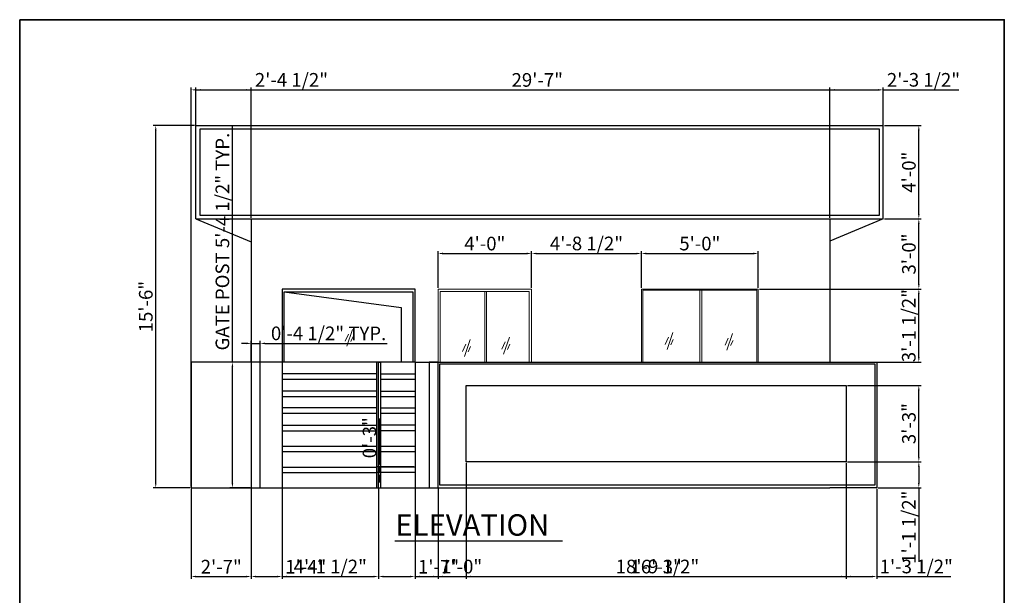
# Model space of a CAD drawing. Units: inches. Extents: x 1484 to 2008, y 1843 to 2590.
# Tile 21 of 21: x 1484 to 1990, y 2295 to 2590. Entities that reach past the tile are written whole.
import ezdxf

# ---------------------------------------------------------------- set-up
doc = ezdxf.new("R2010")
doc.units = ezdxf.units.IN
for name, color, linetype, lineweight in [('A-ANNO-DIMS', 2, 'Continuous', 18), ('A-ANNO-TEXT', 7, 'Continuous', 25), ('A-ANNO-TTLB', 7, 'Continuous', 35), ('A-ELEV', 7, 'Continuous', 30), ('A-ELEV-DOOR', 4, 'Continuous', 25), ('A-ELEV-GATE', 7, 'Continuous', 25), ('A-ELEV-GLAZ', 4, 'Continuous', 18), ('A-ELEV-ROOF', 7, 'Continuous', 30)]:
    doc.layers.add(name, color=color, linetype=linetype, lineweight=lineweight)
doc.styles.get("Standard").update_dxf_attribs({"font": 'arial.ttf'})
doc.dimstyles.new('ISO-25', dxfattribs={"dimtxt": 7, "dimasz": 2.5, "dimexe": 1.25, "dimexo": 0.625, "dimtad": 1, "dimdec": 0, "dimlunit": 3, "dimtxsty": 'Standard', "dimcen": 2.5, "dimadec": 0, "dimazin": 0, "dimtfac": 1, "dimtdec": 0, "dimtmove": 0, "dimatfit": 3, "dimfxl": 1, "dimarcsym": 0})

# ---------------------------------------------------------------- blocks, each defined once
blk = doc.blocks.new('GLASS-REFLECTION')
for p, q in [((1.68, 6.24), (0, 2.6)), ((3.87, 8.69), (0.89, 0)), ((4.11, 5.06), (2.86, 2.41))]:
    blk.add_line(p, q)
blk = doc.blocks.new('GATE-POST-ELEV')
blk.add_lwpolyline([(4.59, 64.44), (0, 64.44), (0, 0), (4.59, 0)], close=True)
blk = doc.blocks.new('*D15')
at = {"layer": 'A-ANNO-DIMS', "color": 0, "lineweight": -2, "transparency": 16777216}
for p, q in [((1593.25, 2414.26), (1593.25, 2535.55)), ((1602.29, 2414.26), (1592, 2414.26)), ((1593.25, 2352.32), (1593.25, 2411.76)), ((1602.29, 2349.82), (1592, 2349.82))]:
    blk.add_line(p, q, dxfattribs=at)
at = {"layer": 'A-ANNO-DIMS', "color": 0, "transparency": 16777216}
for points in [[(1592.84, 2411.76), (1593.67, 2411.76), (1593.25, 2414.26)], [(1592.84, 2352.32), (1593.67, 2352.32), (1593.25, 2349.82)]]:
    blk.add_solid(points, dxfattribs=at)
at = {"layer": 'Defpoints', "color": 0, "transparency": 16777216}
for p in [(1593.25, 2414.26), (1602.92, 2414.26), (1602.92, 2349.82)]:
    blk.add_point(p, dxfattribs=at)
at = {"layer": 'A-ANNO-DIMS', "color": 0, "transparency": 16777216, "insert": (1589.01, 2476.16), "char_height": 7, "attachment_point": 5, "rotation": 90}
blk.add_mtext('GATE POST 5\'-4 1/2" TYP.', dxfattribs=at)
blk = doc.blocks.new('*D16')
at = {"layer": 'A-ANNO-DIMS', "color": 0, "lineweight": -2, "transparency": 16777216}
for p, q in [((1600.42, 2423.92), (1597.92, 2423.92)), ((1602.92, 2414.88), (1602.92, 2425.17)), ((1602.92, 2423.92), (1607.51, 2423.92)), ((1607.51, 2414.88), (1607.51, 2425.17)), ((1610.01, 2423.92), (1672.74, 2423.92))]:
    blk.add_line(p, q, dxfattribs=at)
at = {"layer": 'A-ANNO-DIMS', "color": 0, "transparency": 16777216}
for points in [[(1600.42, 2424.34), (1600.42, 2423.5), (1602.92, 2423.92)], [(1610.01, 2424.34), (1610.01, 2423.5), (1607.51, 2423.92)]]:
    blk.add_solid(points, dxfattribs=at)
at = {"layer": 'Defpoints', "color": 0, "transparency": 16777216}
for p in [(1607.51, 2423.92), (1602.92, 2414.26), (1607.51, 2414.26)]:
    blk.add_point(p, dxfattribs=at)
at = {"layer": 'A-ANNO-DIMS', "color": 0, "transparency": 16777216, "insert": (1642.62, 2428.17), "char_height": 7, "attachment_point": 5}
blk.add_mtext('0\'-4 1/2" TYP.', dxfattribs=at)
blk = doc.blocks.new('*D44')
at = {"layer": 'A-ANNO-DIMS', "color": 0, "lineweight": -2, "transparency": 16777216}
for p, q in [((1572.14, 2350.44), (1572.14, 2555.32)), ((1574.64, 2554.07), (1924.89, 2554.07)), ((1927.39, 2536.44), (1927.39, 2555.32))]:
    blk.add_line(p, q, dxfattribs=at)
at = {"layer": 'A-ANNO-DIMS', "color": 0, "transparency": 16777216}
for points in [[(1574.64, 2554.49), (1574.64, 2553.65), (1572.14, 2554.07)], [(1924.89, 2554.49), (1924.89, 2553.65), (1927.39, 2554.07)]]:
    blk.add_solid(points, dxfattribs=at)
at = {"layer": 'Defpoints', "color": 0, "transparency": 16777216}
for p in [(1927.39, 2554.07), (1927.39, 2535.82), (1572.14, 2349.82)]:
    blk.add_point(p, dxfattribs=at)
at = {"layer": 'A-ANNO-DIMS', "color": 0, "transparency": 16777216, "insert": (1749.76, 2558.27), "char_height": 7, "attachment_point": 5}
blk.add_mtext('29\'-7"', dxfattribs=at)
blk = doc.blocks.new('*D45')
at = {"layer": 'A-ANNO-DIMS', "color": 0, "lineweight": -2, "transparency": 16777216}
for p, q in [((1573.86, 2535.82), (1552.64, 2535.82)), ((1553.89, 2352.32), (1553.89, 2533.32)), ((1571.51, 2349.82), (1552.64, 2349.82))]:
    blk.add_line(p, q, dxfattribs=at)
at = {"layer": 'A-ANNO-DIMS', "color": 0, "transparency": 16777216}
for points in [[(1553.47, 2533.32), (1554.3, 2533.32), (1553.89, 2535.82)], [(1553.47, 2352.32), (1554.3, 2352.32), (1553.89, 2349.82)]]:
    blk.add_solid(points, dxfattribs=at)
at = {"layer": 'Defpoints', "color": 0, "transparency": 16777216}
for p in [(1553.89, 2535.82), (1574.48, 2535.82), (1572.14, 2349.82)]:
    blk.add_point(p, dxfattribs=at)
at = {"layer": 'A-ANNO-DIMS', "color": 0, "transparency": 16777216, "insert": (1549.69, 2442.82), "char_height": 7, "attachment_point": 5, "rotation": 90}
blk.add_mtext('15\'-6"', dxfattribs=at)
blk = doc.blocks.new('*D46')
at = {"layer": 'A-ANNO-DIMS', "color": 0, "lineweight": -2, "transparency": 16777216}
for p, q in [((1574.48, 2488.44), (1574.48, 2555.32)), ((1576.98, 2554.07), (1600.42, 2554.07)), ((1602.92, 2488.44), (1602.92, 2555.32)), ((1602.92, 2554.07), (1641.71, 2554.07))]:
    blk.add_line(p, q, dxfattribs=at)
at = {"layer": 'A-ANNO-DIMS', "color": 0, "transparency": 16777216}
for points in [[(1576.98, 2554.49), (1576.98, 2553.65), (1574.48, 2554.07)], [(1600.42, 2554.49), (1600.42, 2553.65), (1602.92, 2554.07)]]:
    blk.add_solid(points, dxfattribs=at)
at = {"layer": 'Defpoints', "color": 0, "transparency": 16777216}
for p in [(1602.92, 2554.07), (1574.48, 2487.82), (1602.92, 2487.82)]:
    blk.add_point(p, dxfattribs=at)
at = {"layer": 'A-ANNO-DIMS', "color": 0, "transparency": 16777216, "insert": (1623.56, 2558.31), "char_height": 7, "attachment_point": 5}
blk.add_mtext('2\'-4 1/2"', dxfattribs=at)
blk = doc.blocks.new('*D47')
at = {"layer": 'A-ANNO-DIMS', "color": 0, "lineweight": -2, "transparency": 16777216}
for p, q in [((1899.92, 2488.44), (1899.92, 2555.32)), ((1902.42, 2554.07), (1924.89, 2554.07)), ((1927.39, 2488.44), (1927.39, 2555.32)), ((1927.39, 2554.07), (1966.17, 2554.07))]:
    blk.add_line(p, q, dxfattribs=at)
at = {"layer": 'A-ANNO-DIMS', "color": 0, "transparency": 16777216}
for points in [[(1902.42, 2554.49), (1902.42, 2553.65), (1899.92, 2554.07)], [(1924.89, 2554.49), (1924.89, 2553.65), (1927.39, 2554.07)]]:
    blk.add_solid(points, dxfattribs=at)
at = {"layer": 'Defpoints', "color": 0, "transparency": 16777216}
for p in [(1927.39, 2554.07), (1899.92, 2487.82), (1927.39, 2487.82)]:
    blk.add_point(p, dxfattribs=at)
at = {"layer": 'A-ANNO-DIMS', "color": 0, "transparency": 16777216, "insert": (1948.03, 2558.32), "char_height": 7, "attachment_point": 5}
blk.add_mtext('2\'-3 1/2"', dxfattribs=at)
blk = doc.blocks.new('*D48')
at = {"layer": 'A-ANNO-DIMS', "color": 0, "lineweight": -2, "transparency": 16777216}
for p, q in [((1928.01, 2535.82), (1946.89, 2535.82)), ((1945.64, 2490.32), (1945.64, 2533.32)), ((1928.01, 2487.82), (1946.89, 2487.82))]:
    blk.add_line(p, q, dxfattribs=at)
at = {"layer": 'A-ANNO-DIMS', "color": 0, "transparency": 16777216}
for points in [[(1945.22, 2533.32), (1946.05, 2533.32), (1945.64, 2535.82)], [(1945.22, 2490.32), (1946.05, 2490.32), (1945.64, 2487.82)]]:
    blk.add_solid(points, dxfattribs=at)
at = {"layer": 'Defpoints', "color": 0, "transparency": 16777216}
for p in [(1927.39, 2535.82), (1945.64, 2535.82), (1927.39, 2487.82)]:
    blk.add_point(p, dxfattribs=at)
at = {"layer": 'A-ANNO-DIMS', "color": 0, "transparency": 16777216, "insert": (1941.44, 2511.82), "char_height": 7, "attachment_point": 5, "rotation": 90}
blk.add_mtext('4\'-0"', dxfattribs=at)
blk = doc.blocks.new('*D49')
at = {"layer": 'A-ANNO-DIMS', "color": 0, "lineweight": -2, "transparency": 16777216}
for p, q in [((1928.01, 2487.82), (1946.89, 2487.82)), ((1945.64, 2454.32), (1945.64, 2485.32)), ((1863.84, 2451.82), (1946.89, 2451.82))]:
    blk.add_line(p, q, dxfattribs=at)
at = {"layer": 'A-ANNO-DIMS', "color": 0, "transparency": 16777216}
for points in [[(1945.22, 2485.32), (1946.05, 2485.32), (1945.64, 2487.82)], [(1945.22, 2454.32), (1946.05, 2454.32), (1945.64, 2451.82)]]:
    blk.add_solid(points, dxfattribs=at)
at = {"layer": 'Defpoints', "color": 0, "transparency": 16777216}
for p in [(1927.39, 2487.82), (1945.64, 2487.82), (1863.22, 2451.82)]:
    blk.add_point(p, dxfattribs=at)
at = {"layer": 'A-ANNO-DIMS', "color": 0, "transparency": 16777216, "insert": (1941.44, 2469.82), "char_height": 7, "attachment_point": 5, "rotation": 90}
blk.add_mtext('3\'-0"', dxfattribs=at)
blk = doc.blocks.new('*D50')
at = {"layer": 'A-ANNO-DIMS', "color": 0, "lineweight": -2, "transparency": 16777216}
for p, q in [((1863.84, 2451.82), (1946.89, 2451.82)), ((1945.64, 2416.76), (1945.64, 2449.32)), ((1863.84, 2414.26), (1946.89, 2414.26))]:
    blk.add_line(p, q, dxfattribs=at)
at = {"layer": 'A-ANNO-DIMS', "color": 0, "transparency": 16777216}
for points in [[(1945.22, 2449.32), (1946.05, 2449.32), (1945.64, 2451.82)], [(1945.22, 2416.76), (1946.05, 2416.76), (1945.64, 2414.26)]]:
    blk.add_solid(points, dxfattribs=at)
at = {"layer": 'Defpoints', "color": 0, "transparency": 16777216}
for p in [(1863.22, 2451.82), (1945.64, 2451.82), (1863.22, 2414.26)]:
    blk.add_point(p, dxfattribs=at)
at = {"layer": 'A-ANNO-DIMS', "color": 0, "transparency": 16777216, "insert": (1941.39, 2433.04), "char_height": 7, "attachment_point": 5, "rotation": 90}
blk.add_mtext('3\'-1 1/2"', dxfattribs=at)
blk = doc.blocks.new('*D51')
at = {"layer": 'A-ANNO-DIMS', "color": 0, "lineweight": -2, "transparency": 16777216}
for p, q in [((1572.14, 2349.19), (1572.14, 2302.99)), ((1602.92, 2349.19), (1602.92, 2302.99)), ((1574.64, 2304.24), (1600.42, 2304.24))]:
    blk.add_line(p, q, dxfattribs=at)
at = {"layer": 'A-ANNO-DIMS', "color": 0, "transparency": 16777216}
for points in [[(1574.64, 2304.66), (1574.64, 2303.83), (1572.14, 2304.24)], [(1600.42, 2304.66), (1600.42, 2303.83), (1602.92, 2304.24)]]:
    blk.add_solid(points, dxfattribs=at)
at = {"layer": 'Defpoints', "color": 0, "transparency": 16777216}
for p in [(1572.14, 2349.82), (1602.92, 2349.82), (1602.92, 2304.24)]:
    blk.add_point(p, dxfattribs=at)
at = {"layer": 'A-ANNO-DIMS', "color": 0, "transparency": 16777216, "insert": (1587.53, 2308.38), "char_height": 7, "attachment_point": 5}
blk.add_mtext('2\'-7"', dxfattribs=at)
blk = doc.blocks.new('*D52')
at = {"layer": 'A-ANNO-DIMS', "color": 0, "lineweight": -2, "transparency": 16777216}
for p, q in [((1602.92, 2349.19), (1602.92, 2302.99)), ((1618.8, 2349.19), (1618.8, 2302.99)), ((1605.42, 2304.24), (1616.3, 2304.24)), ((1618.8, 2304.24), (1640.49, 2304.24))]:
    blk.add_line(p, q, dxfattribs=at)
at = {"layer": 'A-ANNO-DIMS', "color": 0, "transparency": 16777216}
for points in [[(1605.42, 2304.66), (1605.42, 2303.83), (1602.92, 2304.24)], [(1616.3, 2304.66), (1616.3, 2303.83), (1618.8, 2304.24)]]:
    blk.add_solid(points, dxfattribs=at)
at = {"layer": 'Defpoints', "color": 0, "transparency": 16777216}
for p in [(1602.92, 2349.82), (1618.8, 2349.82), (1618.8, 2304.24)]:
    blk.add_point(p, dxfattribs=at)
at = {"layer": 'A-ANNO-DIMS', "color": 0, "transparency": 16777216, "insert": (1630.89, 2308.38), "char_height": 7, "attachment_point": 5}
blk.add_mtext('1\'-4"', dxfattribs=at)
blk = doc.blocks.new('*D53')
at = {"layer": 'A-ANNO-DIMS', "color": 0, "lineweight": -2, "transparency": 16777216}
for p, q in [((1618.8, 2349.19), (1618.8, 2302.99)), ((1668.22, 2349.19), (1668.22, 2302.99)), ((1621.3, 2304.24), (1665.72, 2304.24))]:
    blk.add_line(p, q, dxfattribs=at)
at = {"layer": 'A-ANNO-DIMS', "color": 0, "transparency": 16777216}
for points in [[(1621.3, 2304.66), (1621.3, 2303.83), (1618.8, 2304.24)], [(1665.72, 2304.66), (1665.72, 2303.83), (1668.22, 2304.24)]]:
    blk.add_solid(points, dxfattribs=at)
at = {"layer": 'Defpoints', "color": 0, "transparency": 16777216}
for p in [(1618.8, 2349.82), (1668.22, 2349.82), (1668.22, 2304.24)]:
    blk.add_point(p, dxfattribs=at)
at = {"layer": 'A-ANNO-DIMS', "color": 0, "transparency": 16777216, "insert": (1643.51, 2308.49), "char_height": 7, "attachment_point": 5}
blk.add_mtext('4\'-1 1/2"', dxfattribs=at)
blk = doc.blocks.new('*D54')
at = {"layer": 'A-ANNO-DIMS', "color": 0, "lineweight": -2, "transparency": 16777216}
for p, q in [((1668.22, 2349.19), (1668.22, 2302.99)), ((1686.99, 2349.19), (1686.99, 2302.99)), ((1670.72, 2304.24), (1684.49, 2304.24)), ((1686.99, 2304.24), (1708.69, 2304.24))]:
    blk.add_line(p, q, dxfattribs=at)
at = {"layer": 'A-ANNO-DIMS', "color": 0, "transparency": 16777216}
for points in [[(1670.72, 2304.66), (1670.72, 2303.83), (1668.22, 2304.24)], [(1684.49, 2304.66), (1684.49, 2303.83), (1686.99, 2304.24)]]:
    blk.add_solid(points, dxfattribs=at)
at = {"layer": 'Defpoints', "color": 0, "transparency": 16777216}
for p in [(1668.22, 2349.82), (1686.99, 2349.82), (1686.99, 2304.24)]:
    blk.add_point(p, dxfattribs=at)
at = {"layer": 'A-ANNO-DIMS', "color": 0, "transparency": 16777216, "insert": (1699.09, 2308.38), "char_height": 7, "attachment_point": 5}
blk.add_mtext('1\'-7"', dxfattribs=at)
blk = doc.blocks.new('*D55')
at = {"layer": 'A-ANNO-DIMS', "color": 0, "lineweight": -2, "transparency": 16777216}
for p, q in [((1686.99, 2349.19), (1686.99, 2302.99)), ((1698.84, 2349.19), (1698.84, 2302.99)), ((1689.49, 2304.24), (1696.34, 2304.24)), ((1698.84, 2304.24), (1720.54, 2304.24))]:
    blk.add_line(p, q, dxfattribs=at)
at = {"layer": 'A-ANNO-DIMS', "color": 0, "transparency": 16777216}
for points in [[(1689.49, 2304.66), (1689.49, 2303.83), (1686.99, 2304.24)], [(1696.34, 2304.66), (1696.34, 2303.83), (1698.84, 2304.24)]]:
    blk.add_solid(points, dxfattribs=at)
at = {"layer": 'Defpoints', "color": 0, "transparency": 16777216}
for p in [(1686.99, 2349.82), (1698.84, 2349.82), (1698.84, 2304.24)]:
    blk.add_point(p, dxfattribs=at)
at = {"layer": 'A-ANNO-DIMS', "color": 0, "transparency": 16777216, "insert": (1710.94, 2308.44), "char_height": 7, "attachment_point": 5}
blk.add_mtext('1\'-0"', dxfattribs=at)
blk = doc.blocks.new('*D56')
at = {"layer": 'A-ANNO-DIMS', "color": 0, "lineweight": -2, "transparency": 16777216}
for p, q in [((1698.84, 2349.19), (1698.84, 2302.99)), ((1924.09, 2349.19), (1924.09, 2302.99)), ((1701.34, 2304.24), (1921.59, 2304.24))]:
    blk.add_line(p, q, dxfattribs=at)
at = {"layer": 'A-ANNO-DIMS', "color": 0, "transparency": 16777216}
for points in [[(1701.34, 2304.66), (1701.34, 2303.83), (1698.84, 2304.24)], [(1921.59, 2304.66), (1921.59, 2303.83), (1924.09, 2304.24)]]:
    blk.add_solid(points, dxfattribs=at)
at = {"layer": 'Defpoints', "color": 0, "transparency": 16777216}
for p in [(1698.84, 2349.82), (1924.09, 2349.82), (1924.09, 2304.24)]:
    blk.add_point(p, dxfattribs=at)
at = {"layer": 'A-ANNO-DIMS', "color": 0, "transparency": 16777216, "insert": (1811.46, 2308.49), "char_height": 7, "attachment_point": 5}
blk.add_mtext('18\'-9 1/2"', dxfattribs=at)
blk = doc.blocks.new('*D57')
at = {"layer": 'A-ANNO-DIMS', "color": 0, "lineweight": -2, "transparency": 16777216}
for p, q in [((1713.22, 2362.56), (1713.22, 2302.99)), ((1908.35, 2362.56), (1908.35, 2302.99)), ((1715.72, 2304.24), (1905.85, 2304.24))]:
    blk.add_line(p, q, dxfattribs=at)
at = {"layer": 'A-ANNO-DIMS', "color": 0, "transparency": 16777216}
for points in [[(1715.72, 2304.66), (1715.72, 2303.83), (1713.22, 2304.24)], [(1905.85, 2304.66), (1905.85, 2303.83), (1908.35, 2304.24)]]:
    blk.add_solid(points, dxfattribs=at)
at = {"layer": 'Defpoints', "color": 0, "transparency": 16777216}
for p in [(1713.22, 2363.18), (1908.35, 2363.18), (1908.35, 2304.24)]:
    blk.add_point(p, dxfattribs=at)
at = {"layer": 'A-ANNO-DIMS', "color": 0, "transparency": 16777216, "insert": (1810.79, 2308.45), "char_height": 7, "attachment_point": 5}
blk.add_mtext('16\'-3"', dxfattribs=at)
blk = doc.blocks.new('*D58')
at = {"layer": 'A-ANNO-DIMS', "color": 0, "lineweight": -2, "transparency": 16777216}
for p, q in [((1908.98, 2402.29), (1946.89, 2402.29)), ((1945.64, 2365.68), (1945.64, 2399.79)), ((1908.98, 2363.18), (1946.89, 2363.18))]:
    blk.add_line(p, q, dxfattribs=at)
at = {"layer": 'A-ANNO-DIMS', "color": 0, "transparency": 16777216}
for points in [[(1945.22, 2399.79), (1946.05, 2399.79), (1945.64, 2402.29)], [(1945.22, 2365.68), (1946.05, 2365.68), (1945.64, 2363.18)]]:
    blk.add_solid(points, dxfattribs=at)
at = {"layer": 'Defpoints', "color": 0, "transparency": 16777216}
for p in [(1908.35, 2402.29), (1945.64, 2402.29), (1908.35, 2363.18)]:
    blk.add_point(p, dxfattribs=at)
at = {"layer": 'A-ANNO-DIMS', "color": 0, "transparency": 16777216, "insert": (1941.44, 2382.74), "char_height": 7, "attachment_point": 5, "rotation": 90}
blk.add_mtext('3\'-3"', dxfattribs=at)
blk = doc.blocks.new('*D59')
at = {"layer": 'A-ANNO-DIMS', "color": 0, "lineweight": -2, "transparency": 16777216}
for p, q in [((1908.98, 2363.18), (1946.89, 2363.18)), ((1945.64, 2360.68), (1945.64, 2352.32)), ((1924.71, 2349.82), (1946.89, 2349.82)), ((1945.64, 2349.82), (1945.64, 2311.81))]:
    blk.add_line(p, q, dxfattribs=at)
at = {"layer": 'A-ANNO-DIMS', "color": 0, "transparency": 16777216}
for points in [[(1945.22, 2360.68), (1946.05, 2360.68), (1945.64, 2363.18)], [(1945.22, 2352.32), (1946.05, 2352.32), (1945.64, 2349.82)]]:
    blk.add_solid(points, dxfattribs=at)
at = {"layer": 'Defpoints', "color": 0, "transparency": 16777216}
for p in [(1908.35, 2363.18), (1924.09, 2349.82), (1945.64, 2349.82)]:
    blk.add_point(p, dxfattribs=at)
at = {"layer": 'A-ANNO-DIMS', "color": 0, "transparency": 16777216, "insert": (1941.39, 2329.56), "char_height": 7, "attachment_point": 5, "rotation": 90}
blk.add_mtext('1\'-1 1/2"', dxfattribs=at)
blk = doc.blocks.new('*D60')
at = {"layer": 'A-ANNO-DIMS', "color": 0, "lineweight": -2, "transparency": 16777216}
for p, q in [((1908.35, 2362.56), (1908.35, 2302.99)), ((1924.09, 2349.19), (1924.09, 2302.99)), ((1910.85, 2304.24), (1921.59, 2304.24)), ((1924.09, 2304.24), (1962.1, 2304.24))]:
    blk.add_line(p, q, dxfattribs=at)
at = {"layer": 'A-ANNO-DIMS', "color": 0, "transparency": 16777216}
for points in [[(1910.85, 2304.66), (1910.85, 2303.83), (1908.35, 2304.24)], [(1921.59, 2304.66), (1921.59, 2303.83), (1924.09, 2304.24)]]:
    blk.add_solid(points, dxfattribs=at)
at = {"layer": 'Defpoints', "color": 0, "transparency": 16777216}
for p in [(1908.35, 2363.18), (1924.09, 2349.82), (1924.09, 2304.24)]:
    blk.add_point(p, dxfattribs=at)
at = {"layer": 'A-ANNO-DIMS', "color": 0, "transparency": 16777216, "insert": (1944.34, 2308.49), "char_height": 7, "attachment_point": 5}
blk.add_mtext('1\'-3 1/2"', dxfattribs=at)
blk = doc.blocks.new('*D61')
at = {"layer": 'A-ANNO-DIMS', "color": 0, "lineweight": -2, "transparency": 16777216}
for p, q in [((1698.84, 2452.44), (1698.84, 2471.32)), ((1701.34, 2470.07), (1744.34, 2470.07)), ((1746.84, 2452.44), (1746.84, 2471.32))]:
    blk.add_line(p, q, dxfattribs=at)
at = {"layer": 'A-ANNO-DIMS', "color": 0, "transparency": 16777216}
for points in [[(1701.34, 2470.49), (1701.34, 2469.65), (1698.84, 2470.07)], [(1744.34, 2470.49), (1744.34, 2469.65), (1746.84, 2470.07)]]:
    blk.add_solid(points, dxfattribs=at)
at = {"layer": 'Defpoints', "color": 0, "transparency": 16777216}
for p in [(1746.84, 2470.07), (1698.84, 2451.82), (1746.84, 2451.82)]:
    blk.add_point(p, dxfattribs=at)
at = {"layer": 'A-ANNO-DIMS', "color": 0, "transparency": 16777216, "insert": (1722.84, 2474.27), "char_height": 7, "attachment_point": 5}
blk.add_mtext('4\'-0"', dxfattribs=at)
blk = doc.blocks.new('*D62')
at = {"layer": 'A-ANNO-DIMS', "color": 0, "lineweight": -2, "transparency": 16777216}
for p, q in [((1746.84, 2452.44), (1746.84, 2471.32)), ((1749.34, 2470.07), (1800.72, 2470.07)), ((1803.22, 2452.44), (1803.22, 2471.32))]:
    blk.add_line(p, q, dxfattribs=at)
at = {"layer": 'A-ANNO-DIMS', "color": 0, "transparency": 16777216}
for points in [[(1749.34, 2470.49), (1749.34, 2469.65), (1746.84, 2470.07)], [(1800.72, 2470.49), (1800.72, 2469.65), (1803.22, 2470.07)]]:
    blk.add_solid(points, dxfattribs=at)
at = {"layer": 'Defpoints', "color": 0, "transparency": 16777216}
for p in [(1803.22, 2470.07), (1746.84, 2451.82), (1803.22, 2451.82)]:
    blk.add_point(p, dxfattribs=at)
at = {"layer": 'A-ANNO-DIMS', "color": 0, "transparency": 16777216, "insert": (1775.03, 2474.31), "char_height": 7, "attachment_point": 5}
blk.add_mtext('4\'-8 1/2"', dxfattribs=at)
blk = doc.blocks.new('*D63')
at = {"layer": 'A-ANNO-DIMS', "color": 0, "lineweight": -2, "transparency": 16777216}
for p, q in [((1803.22, 2452.44), (1803.22, 2471.32)), ((1805.72, 2470.07), (1860.72, 2470.07)), ((1863.22, 2452.44), (1863.22, 2471.32))]:
    blk.add_line(p, q, dxfattribs=at)
at = {"layer": 'A-ANNO-DIMS', "color": 0, "transparency": 16777216}
for points in [[(1805.72, 2470.49), (1805.72, 2469.65), (1803.22, 2470.07)], [(1860.72, 2470.49), (1860.72, 2469.65), (1863.22, 2470.07)]]:
    blk.add_solid(points, dxfattribs=at)
at = {"layer": 'Defpoints', "color": 0, "transparency": 16777216}
for p in [(1863.22, 2470.07), (1803.22, 2451.82), (1863.22, 2451.82)]:
    blk.add_point(p, dxfattribs=at)
at = {"layer": 'A-ANNO-DIMS', "color": 0, "transparency": 16777216, "insert": (1833.22, 2474.27), "char_height": 7, "attachment_point": 5}
blk.add_mtext('5\'-0"', dxfattribs=at)
blk = doc.blocks.new('*D64')
at = {"layer": 'A-ANNO-DIMS', "color": 0, "lineweight": -2, "transparency": 16777216}
for p, q in [((1668.74, 2363.07), (1668.74, 2385.42)), ((1686.37, 2360.57), (1667.49, 2360.57)), ((1686.37, 2357.57), (1667.49, 2357.57)), ((1668.74, 2357.57), (1668.74, 2360.57)), ((1668.74, 2355.07), (1668.74, 2352.57))]:
    blk.add_line(p, q, dxfattribs=at)
at = {"layer": 'A-ANNO-DIMS', "color": 0, "transparency": 16777216}
for points in [[(1668.33, 2363.07), (1669.16, 2363.07), (1668.74, 2360.57)], [(1668.33, 2355.07), (1669.16, 2355.07), (1668.74, 2357.57)]]:
    blk.add_solid(points, dxfattribs=at)
at = {"layer": 'Defpoints', "color": 0, "transparency": 16777216}
for p in [(1668.74, 2360.57), (1686.99, 2360.57), (1686.99, 2357.57)]:
    blk.add_point(p, dxfattribs=at)
at = {"layer": 'A-ANNO-DIMS', "color": 0, "transparency": 16777216, "insert": (1664.54, 2375.5), "char_height": 7, "attachment_point": 5, "rotation": 90}
blk.add_mtext('0\'-3"', dxfattribs=at)

msp = doc.modelspace()

# ---------------------------------------------------------------- linework, layer by layer
at = {"layer": 'A-ANNO-TEXT'}
msp.add_line((1676.67, 2322.49), (1762.74, 2322.49), dxfattribs=at)
at = {"layer": 'A-ANNO-TTLB'}
msp.add_lwpolyline([(1484.04, 2590.09), (1989.53, 2590.09), (1989.53, 1843.34), (1484.04, 1843.34)], close=True, dxfattribs=at)
at = {"layer": 'A-ELEV'}
for p, q in [((1602.92, 2487.82), (1602.92, 2414.26)), ((1899.92, 2487.82), (1899.92, 2414.26)), ((1686.99, 2414.26), (1572.14, 2414.26)), ((1572.14, 2414.26), (1572.14, 2349.82)), ((1686.99, 2414.26), (1924.09, 2414.26)), ((1924.09, 2414.26), (1924.09, 2349.82)), ((1572.14, 2349.82), (1602.92, 2349.82)), ((1602.92, 2349.82), (1899.92, 2349.82)), ((1924.09, 2349.82), (1899.92, 2349.82))]:
    msp.add_line(p, q, dxfattribs=at)
for points in [[(1699.72, 2413.49), (1923.01, 2413.49), (1923.01, 2351.09), (1699.72, 2351.09)], [(1713.22, 2402.29), (1908.35, 2402.29), (1908.35, 2363.18), (1713.22, 2363.18)]]:
    msp.add_lwpolyline(points, close=True, dxfattribs=at)
at = {"layer": 'A-ELEV-DOOR'}
for p, q in [((1686.99, 2451.82), (1618.8, 2451.82)), ((1618.8, 2451.82), (1618.8, 2414.26)), ((1686.99, 2414.26), (1686.99, 2451.82)), ((1619.78, 2450.44), (1679.8, 2442.42)), ((1679.8, 2442.42), (1679.8, 2414.26))]:
    msp.add_line(p, q, dxfattribs=at)
msp.add_lwpolyline([(1619.78, 2450.44), (1685.79, 2450.44), (1685.79, 2414.26), (1619.78, 2414.26)], close=True, dxfattribs=at)
at = {"layer": 'A-ELEV-GATE'}
for p, q in [((1618.8, 2414.26), (1618.8, 2367.82)), ((1618.8, 2414.26), (1618.8, 2349.82)), ((1667.22, 2414.26), (1667.22, 2349.82)), ((1668.22, 2349.82), (1668.22, 2414.26)), ((1668.22, 2414.26), (1669.22, 2414.26)), ((1669.22, 2414.26), (1669.22, 2349.82)), ((1686.99, 2414.26), (1686.99, 2367.82)), ((1686.99, 2414.26), (1686.99, 2349.82)), ((1618.8, 2408.41), (1667.22, 2408.41)), ((1667.22, 2408.41), (1667.22, 2405.41)), ((1669.22, 2408.38), (1686.99, 2408.38)), ((1686.99, 2408.38), (1686.99, 2405.38)), ((1667.22, 2405.41), (1618.8, 2405.41)), ((1686.99, 2405.38), (1669.22, 2405.38)), ((1618.8, 2399.53), (1667.22, 2399.53)), ((1667.22, 2396.53), (1618.8, 2396.53)), ((1669.22, 2399.45), (1686.99, 2399.45)), ((1686.99, 2396.45), (1669.22, 2396.45)), ((1618.8, 2390.94), (1667.22, 2390.94)), ((1667.22, 2387.94), (1618.8, 2387.94)), ((1669.22, 2390.88), (1686.99, 2390.88)), ((1686.99, 2387.88), (1669.22, 2387.88)), ((1618.8, 2381.9), (1667.22, 2381.9)), ((1669.22, 2382.04), (1686.99, 2382.04)), ((1667.22, 2378.9), (1618.8, 2378.9)), ((1686.99, 2379.04), (1669.22, 2379.04)), ((1618.8, 2371.21), (1667.22, 2371.21)), ((1669.22, 2371.23), (1686.99, 2371.23)), ((1667.22, 2368.21), (1618.8, 2368.21)), ((1686.99, 2368.23), (1669.22, 2368.23)), ((1618.8, 2360.47), (1667.22, 2360.47)), ((1667.22, 2357.47), (1618.8, 2357.47)), ((1669.22, 2360.57), (1686.99, 2360.57)), ((1686.99, 2357.57), (1669.22, 2357.57)), ((1667.22, 2349.82), (1668.22, 2349.82))]:
    msp.add_line(p, q, dxfattribs=at)
at = {"layer": 'A-ELEV-GLAZ'}
for p, q in [((1698.84, 2451.82), (1698.84, 2414.26)), ((1698.84, 2451.82), (1746.84, 2451.82)), ((1746.84, 2451.82), (1746.84, 2414.26)), ((1803.22, 2451.82), (1803.22, 2414.26)), ((1803.22, 2451.82), (1863.22, 2451.82)), ((1863.22, 2451.82), (1863.22, 2414.26)), ((1722.76, 2450.54), (1722.76, 2414.26)), ((1723.76, 2414.26), (1723.76, 2450.54)), ((1833.25, 2451.23), (1833.25, 2414.26)), ((1834.25, 2414.26), (1834.25, 2451.23))]:
    msp.add_line(p, q, dxfattribs=at)
for points in [[(1699.96, 2414.26), (1699.96, 2450.54), (1745.56, 2450.54), (1745.56, 2414.26)], [(1804, 2414.26), (1804, 2451.23), (1862.5, 2451.23), (1862.5, 2414.26)]]:
    msp.add_lwpolyline(points, dxfattribs=at)
at = {"layer": 'A-ELEV-ROOF'}
for p, q in [((1574.48, 2535.82), (1927.39, 2535.82)), ((1574.48, 2487.82), (1574.48, 2535.82)), ((1925.39, 2533.82), (1576.48, 2533.82)), ((1576.48, 2533.82), (1576.48, 2489.82)), ((1925.39, 2489.82), (1925.39, 2533.82)), ((1927.39, 2487.82), (1927.39, 2535.82)), ((1574.48, 2487.82), (1574.48, 2489.82)), ((1574.48, 2487.82), (1927.39, 2487.82)), ((1574.48, 2487.82), (1602.92, 2476.14)), ((1576.48, 2489.82), (1925.39, 2489.82)), ((1927.39, 2487.82), (1899.92, 2476.33)), ((1899.92, 2476.33), (1899.92, 2476.33))]:
    msp.add_line(p, q, dxfattribs=at)

# ---------------------------------------------------------------- block references
at = {"layer": 'A-ELEV'}
for p in [(1602.92, 2349.82), (1694.25, 2349.82)]:
    msp.add_blockref('GATE-POST-ELEV', p, dxfattribs=at)
at = {"layer": 'A-ELEV-GLAZ'}
for p in [(1651.1, 2422.42), (1731.57, 2418.43), (1815.49, 2420.81), (1846.15, 2420.39), (1711.45, 2417.23)]:
    msp.add_blockref('GLASS-REFLECTION', p, dxfattribs=at)

# ---------------------------------------------------------------- texts
at = {"layer": 'A-ANNO-TEXT', "insert": (1676.97, 2336.2), "char_height": 11, "attachment_point": 1}
msp.add_mtext_dynamic_manual_height_columns('ELEVATION', width=217.7638, gutter_width=12.5, heights=[0], dxfattribs=at)

# ---------------------------------------------------------------- dimensions: what is measured, and where the dimension line sits
at = {"layer": 'A-ANNO-DIMS'}
for base, p1, p2, picture, middle in [((1602.92, 2554.07), (1574.48, 2487.82), (1602.92, 2487.82), '*D46', (1623.56, 2558.31)), ((1927.39, 2554.07), (1899.92, 2487.82), (1927.39, 2487.82), '*D47', (1948.03, 2558.32)), ((1927.3866, 2554.0686), (1572.1374, 2349.8186), (1927.3866, 2535.8186), '*D44', (1749.762, 2558.2676)), ((1803.22, 2470.07), (1746.84, 2451.82), (1803.22, 2451.82), '*D62', (1775.03, 2474.31)), ((1746.84, 2470.07), (1698.84, 2451.82), (1746.84, 2451.82), '*D61', (1722.84, 2474.27)), ((1863.22, 2470.07), (1803.22, 2451.82), (1863.22, 2451.82), '*D63', (1833.22, 2474.27)), ((1908.35, 2304.24), (1713.22, 2363.18), (1908.35, 2363.18), '*D57', (1810.79, 2308.45)), ((1924.09, 2304.24), (1908.35, 2363.18), (1924.09, 2349.82), '*D60', (1944.34, 2308.49)), ((1602.92, 2304.24), (1572.14, 2349.82), (1602.92, 2349.82), '*D51', (1587.53, 2308.38)), ((1618.8, 2304.24), (1602.92, 2349.82), (1618.8, 2349.82), '*D52', (1630.89, 2308.38)), ((1668.22, 2304.24), (1618.8, 2349.82), (1668.22, 2349.82), '*D53', (1643.51, 2308.49)), ((1686.99, 2304.24), (1668.22, 2349.82), (1686.99, 2349.82), '*D54', (1699.09, 2308.38)), ((1698.8368, 2304.2444), (1686.9925, 2349.8186), (1698.8368, 2349.8186), '*D55', (1710.9362, 2308.4434)), ((1924.0874, 2304.2444), (1698.8368, 2349.8186), (1924.0874, 2349.8186), '*D56', (1811.4621, 2308.4887))]:
    dim = msp.add_linear_dim(base=base, p1=p1, p2=p2, dimstyle='ISO-25', override={"dimdec": 1, "dimlfac": 1, "dimrnd": 0, "dimzin": 1, "dimdsep": 46, "dimlunit": 4, "dimfrac": 2}, dxfattribs=at)
    dim.commit()
    dim.dimension.update_dxf_attribs({"geometry": picture, "text_midpoint": middle})
for base, p1, p2, picture, middle in [((1553.89, 2535.82), (1572.14, 2349.82), (1574.48, 2535.82), '*D45', (1549.69, 2442.82)), ((1945.64, 2535.82), (1927.39, 2487.82), (1927.39, 2535.82), '*D48', (1941.44, 2511.82)), ((1945.64, 2487.82), (1863.22, 2451.82), (1927.39, 2487.82), '*D49', (1941.44, 2469.82)), ((1945.64, 2451.82), (1863.22, 2414.26), (1863.22, 2451.82), '*D50', (1941.39, 2433.04)), ((1945.64, 2402.29), (1908.35, 2363.18), (1908.35, 2402.29), '*D58', (1941.44, 2382.74)), ((1668.74, 2360.57), (1686.99, 2357.57), (1686.99, 2360.57), '*D64', (1664.54, 2375.5)), ((1945.64, 2349.82), (1908.35, 2363.18), (1924.09, 2349.82), '*D59', (1941.39, 2329.56))]:
    dim = msp.add_linear_dim(base=base, p1=p1, p2=p2, angle=90, dimstyle='ISO-25', override={"dimdec": 1, "dimlfac": 1, "dimrnd": 0, "dimzin": 1, "dimdsep": 46, "dimlunit": 4, "dimfrac": 2}, dxfattribs=at)
    dim.commit()
    dim.dimension.update_dxf_attribs({"geometry": picture, "text_midpoint": middle})
dim = msp.add_linear_dim(base=(1593.25, 2414.26), p1=(1602.92, 2349.82), p2=(1602.92, 2414.26), angle=90, text='GATE POST <> TYP.', dimstyle='ISO-25', override={"dimdec": 1, "dimlfac": 1, "dimrnd": 0, "dimzin": 1, "dimdsep": 46, "dimlunit": 4, "dimfrac": 2}, dxfattribs=at)
dim.commit()
dim.dimension.update_dxf_attribs({"geometry": '*D15', "text_midpoint": (1589.01, 2476.16)})
dim = msp.add_linear_dim(base=(1607.51, 2423.92), p1=(1602.92, 2414.26), p2=(1607.51, 2414.26), text='<> TYP.', dimstyle='ISO-25', override={"dimdec": 1, "dimlfac": 1, "dimrnd": 0, "dimzin": 1, "dimdsep": 46, "dimlunit": 4, "dimfrac": 2}, dxfattribs=at)
dim.commit()
dim.dimension.update_dxf_attribs({"geometry": '*D16', "text_midpoint": (1642.62, 2428.17)})

doc.saveas('drawing.dxf')
